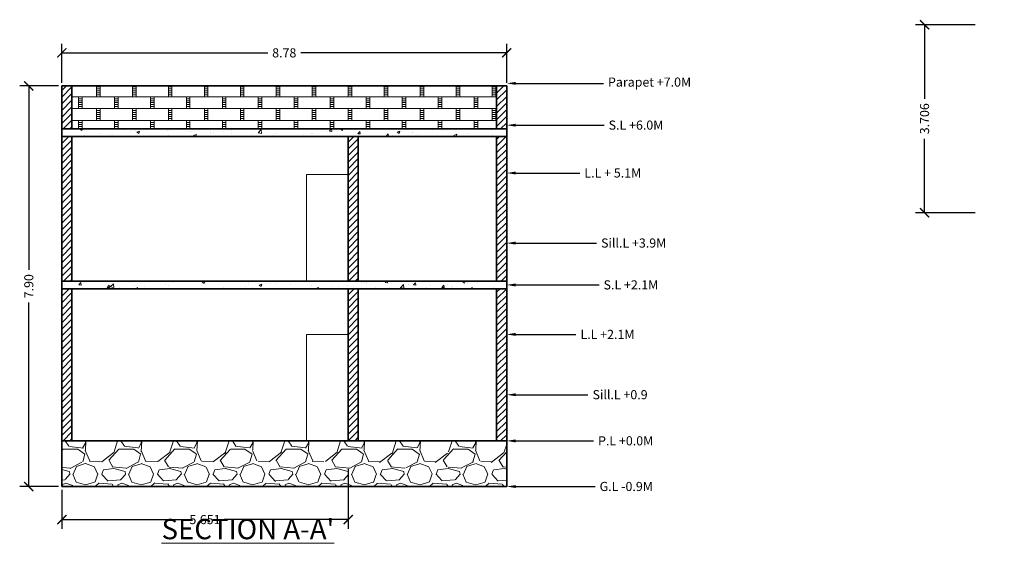
# Model space of a CAD drawing. Units: metres. Extents: x 6.8 to 74, y 0.6 to 37.
# Tile 4 of 5: x 20.7 to 40.1, y 19.5 to 29.9. Entities that reach past the tile are written whole.
import ezdxf
from ezdxf import colors
from ezdxf.entities.mleader import LeaderData, LeaderLine
from ezdxf.math import Vec2, Vec3

# ---------------------------------------------------------------- set-up
doc = ezdxf.new("R2010")
doc.units = ezdxf.units.M
doc.header["$LTSCALE"] = 0.2
doc.header["$MEASUREMENT"] = 0
for name, color, linetype, lineweight in [('A-ANNO-DIMS', 2, 'Continuous', 18), ('A-ANNO-SYMB', 3, 'Continuous', 18), ('A-ANNO-TEXT', 7, 'Continuous', 18), ('A-DOOR', 4, 'Continuous', 20), ('A-SECT', 7, 'Continuous', 35), ('A-SECT-PATT', 252, 'Continuous', 13)]:
    doc.layers.add(name, color=color, linetype=linetype, lineweight=lineweight)
doc.styles.get("Standard").update_dxf_attribs({"font": 'arial.ttf'})
doc.dimstyles.get("Standard").update_dxf_attribs({"dimtxt": 0.18, "dimasz": 0.18, "dimexe": 0.18, "dimexo": 0.0625, "dimgap": 0.09, "dimtad": 0, "dimzin": 0, "dimdsep": 46, "dimtxsty": 'Standard', "dimblk": 'ARCHTICK', "dimcen": 0.09, "dimadec": 0, "dimazin": 0, "dimtfac": 1, "dimtofl": 0, "dimtmove": 0, "dimatfit": 3, "dimfxl": 1, "dimfxlon": 1, "dimtolj": 1, "dimtzin": 0, "dimarcsym": 0})
pattern_1 = [(45, (0, 0), (-0.0654073772597557, 0.0654073772597557), [])]

# ---------------------------------------------------------------- blocks, each defined once
blk = doc.blocks.new('_ArchTick')
at = {"color": 0, "linetype": 'ByBlock', "const_width": 0.15}
blk.add_lwpolyline([(-0.5, -0.5), (0.5, 0.5)], dxfattribs=at)
blk = doc.blocks.new('*D56')
at = {"layer": 'A-ANNO-DIMS', "color": 0, "lineweight": -2, "ltscale": 0.9, "transparency": 16777216}
for p, q in [((21.540083, 28.626551), (21.540083, 29.395551)), ((30.320083, 28.626551), (30.320083, 29.395551)), ((21.540083, 29.215551), (25.60599705184175, 29.215551)), ((30.320083, 29.215551), (26.25416894815825, 29.215551))]:
    blk.add_line(p, q, dxfattribs=at)
at = {"layer": 'Defpoints', "color": 0, "ltscale": 0.9, "transparency": 16777216}
for p in [(30.320083, 29.215551), (21.540083, 28.564051), (30.320083, 28.564051)]:
    blk.add_point(p, dxfattribs=at)
at = {"layer": 'A-ANNO-DIMS', "color": 0, "lineweight": -2, "ltscale": 0.9, "transparency": 16777216, "xscale": 0.18, "yscale": 0.18, "zscale": 0.18, "rotation": 180}
blk.add_blockref('_ArchTick', (21.540083, 29.215551), dxfattribs=at)
at = {"layer": 'A-ANNO-DIMS', "color": 0, "lineweight": -2, "ltscale": 0.9, "transparency": 16777216, "xscale": 0.18, "yscale": 0.18, "zscale": 0.18}
blk.add_blockref('_ArchTick', (30.320083, 29.215551), dxfattribs=at)
at = {"layer": 'A-ANNO-DIMS', "color": 0, "ltscale": 0.9, "transparency": 16777216, "insert": (25.930083, 29.215551), "char_height": 0.18, "attachment_point": 5}
blk.add_mtext('\\A1;8.78', dxfattribs=at)
blk = doc.blocks.new('*D57')
at = {"layer": 'A-ANNO-DIMS', "color": 0, "lineweight": -2, "ltscale": 0.9, "transparency": 16777216}
for p, q in [((21.47758300000001, 28.56405100000002), (20.70858300000002, 28.56405100000002)), ((20.88858300000001, 28.56405100000002), (20.88858300000001, 24.93678633424285)), ((20.88858300000002, 20.66405100000001), (20.88858300000001, 24.29131566575718)), ((21.47758300000001, 20.66405100000001), (20.70858300000002, 20.66405100000001))]:
    blk.add_line(p, q, dxfattribs=at)
at = {"layer": 'Defpoints', "color": 0, "ltscale": 0.9, "transparency": 16777216}
for p in [(20.88858300000001, 28.56405100000002), (21.540083, 28.56405100000002), (21.540083, 20.66405100000001)]:
    blk.add_point(p, dxfattribs=at)
at = {"layer": 'A-ANNO-DIMS', "color": 0, "lineweight": -2, "ltscale": 0.9, "transparency": 16777216, "xscale": 0.18, "yscale": 0.18, "zscale": 0.18}
for p, rotation in [((20.88858300000001, 28.56405100000002), 90), ((20.88858300000002, 20.66405100000001), 270)]:
    blk.add_blockref('_ArchTick', p, dxfattribs=dict(at, rotation=rotation))
at = {"layer": 'A-ANNO-DIMS', "color": 0, "ltscale": 0.9, "transparency": 16777216, "insert": (20.88858300000002, 24.614051), "char_height": 0.18, "attachment_point": 5, "rotation": 90}
blk.add_mtext('\\A1;7.90', dxfattribs=at)
blk = doc.blocks.new('*D58')
at = {"layer": 'A-ANNO-DIMS', "color": 0, "lineweight": -2, "ltscale": 0.9, "transparency": 16777216}
for p, q in [((27.190671, 21.012551), (27.190671, 19.832551)), ((21.540083, 20.601551), (21.540083, 19.832551)), ((21.540083, 20.012551), (23.98904684993178, 20.012551)), ((27.190671, 20.012551), (24.74170715006821, 20.012551))]:
    blk.add_line(p, q, dxfattribs=at)
at = {"layer": 'Defpoints', "color": 0, "ltscale": 0.9, "transparency": 16777216}
for p in [(27.190671, 21.564051), (21.540083, 20.664051), (27.190671, 20.012551)]:
    blk.add_point(p, dxfattribs=at)
at = {"layer": 'A-ANNO-DIMS', "color": 0, "lineweight": -2, "ltscale": 0.9, "transparency": 16777216, "xscale": 0.18, "yscale": 0.18, "zscale": 0.18, "rotation": 180}
blk.add_blockref('_ArchTick', (21.540083, 20.012551), dxfattribs=at)
at = {"layer": 'A-ANNO-DIMS', "color": 0, "lineweight": -2, "ltscale": 0.9, "transparency": 16777216, "xscale": 0.18, "yscale": 0.18, "zscale": 0.18}
blk.add_blockref('_ArchTick', (27.190671, 20.012551), dxfattribs=at)
at = {"layer": 'A-ANNO-DIMS', "color": 0, "ltscale": 0.9, "transparency": 16777216, "insert": (24.365377, 20.012551), "char_height": 0.18, "attachment_point": 5}
blk.add_mtext('\\A1;5.651', dxfattribs=at)
blk = doc.blocks.new('*D61')
at = {"layer": 'A-ANNO-DIMS', "color": 0, "lineweight": -2, "ltscale": 0.9, "transparency": 16777216}
for p, q in [((39.56668000000003, 29.76942700000001), (38.38668000000003, 29.76942700000001)), ((38.56668000000003, 29.76942700000001), (38.56668000000003, 28.30996317326059)), ((38.56668000000003, 26.06333700000001), (38.56668000000003, 27.52280082673944)), ((39.56668000000003, 26.06333700000001), (38.38668000000003, 26.06333700000001))]:
    blk.add_line(p, q, dxfattribs=at)
at = {"layer": 'Defpoints', "color": 0, "ltscale": 0.9, "transparency": 16777216}
for p in [(38.56668000000003, 29.76942700000001), (52.66698100000002, 29.76942700000002), (52.66698100000002, 26.06333700000002)]:
    blk.add_point(p, dxfattribs=at)
at = {"layer": 'A-ANNO-DIMS', "color": 0, "lineweight": -2, "ltscale": 0.9, "transparency": 16777216, "xscale": 0.18, "yscale": 0.18, "zscale": 0.18}
for p, rotation in [((38.56668000000003, 29.76942700000001), 90), ((38.56668000000003, 26.06333700000001), 270)]:
    blk.add_blockref('_ArchTick', p, dxfattribs=dict(at, rotation=rotation))
at = {"layer": 'A-ANNO-DIMS', "color": 0, "ltscale": 0.9, "transparency": 16777216, "insert": (38.56668000000003, 27.91638199999999), "char_height": 0.18, "attachment_point": 5, "rotation": 90}
blk.add_mtext('\\A1;3.706', dxfattribs=at)

msp = doc.modelspace()

# ---------------------------------------------------------------- hatches: boundary and pattern name
at = {"layer": 'A-SECT-PATT'}
h = msp.add_hatch(dxfattribs=at)
h.set_pattern_fill('ANSI31', color=256, scale=0.7400000000000001)
h.set_pattern_definition(pattern_1)
h.paths.add_polyline_path([(21.7400830914722, 27.56405142054635), (21.5400830914722, 27.56405142054635), (21.5400830914722, 24.71405142054635), (21.7400830914722, 24.71405142054635)])
h.paths.add_polyline_path([(21.7400830914722, 28.56405142054635), (21.5400830914722, 28.56405142054635), (21.5400830914722, 27.71405142054635), (21.7400830914722, 27.71405142054635)])
h.paths.add_polyline_path([(30.32008309147219, 28.56405142054635), (30.1200830914722, 28.56405142054635), (30.1200830914722, 27.71405142054635), (30.3200830914722, 27.71405142054635)])
h.paths.add_polyline_path([(30.3200830914722, 27.56405142054635), (30.1200830914722, 27.56405142054635), (30.1200830914722, 24.71405142054635), (30.3200830914722, 24.71405142054635)])
h.paths.add_polyline_path([(21.7400830914722, 24.56405142054635), (21.5400830914722, 24.56405142054635), (21.5400830914722, 21.56405142054635), (21.7400830914722, 21.56405142054635)])
h.paths.add_polyline_path([(30.3200830914722, 24.56405142054635), (30.1200830914722, 24.56405142054635), (30.1200830914722, 21.56405142054635), (30.3200830914722, 21.56405142054635)])
h = msp.add_hatch(dxfattribs=at)
h.set_pattern_fill('BRSTONE', color=256, scale=0.71)
h.set_pattern_definition([(0, (0, 0), (0, 0.2343), []), (90, (0.6390000000000001, 0), (-0.355, 0.2343), [0.2343, -0.2343]), (90, (0.568, 0), (-0.355, 0.2343), [0.2343, -0.2343]), (0, (0.6390000000000001, 0.03905), (0.355, 0.2343), [-0.6390000000000001, 0.071]), (0, (0.6390000000000001, 0.0781), (0.355, 0.2343), [-0.6390000000000001, 0.071]), (0, (0.6390000000000001, 0.11715), (0.355, 0.2343), [-0.6390000000000001, 0.071]), (0, (0.6390000000000001, 0.1562), (0.355, 0.2343), [-0.6390000000000001, 0.071]), (0, (0.6390000000000001, 0.19525), (0.355, 0.2343), [-0.6390000000000001, 0.071])])
h.paths.add_polyline_path([(30.1200830914722, 28.56405142054635), (21.7400830914722, 28.56405142054635), (21.7400830914722, 27.71405142054635), (30.1200830914722, 27.71405142054635)])
h = msp.add_hatch(dxfattribs=at)
h.set_pattern_fill('AR-CONC', color=256, scale=0.078)
h.set_pattern_definition([(50, (0, 0), (0.5594629424285877, -0.0489466652864242), [0.0585, -0.6435]), (355, (0, 0), (-0.10822604021814, 0.5867098642860094), [0.0468, -0.5148]), (100.45144446, (0.04662191118, -0.00407888832), (0.4512369004471474, 0.537763192955531), [0.04971734976, -0.5468908473599999]), (46.1842, (0, 0.156), (0.8324482379238265, -0.1291050390185997), [0.08775, -0.9652499999999999]), (96.63563549000003, (0.0693706611, 0.14524122054), (0.7290363176258982, 0.7598125086041494), [0.07457606676, -0.8203367327999997]), (351.18416399, (0, 0.156), (0.729036317142723, 0.7598125082105924), [0.0702, -0.77220000078]), (21, (0.078, 0.117), (0.4655875006524001, -0.3140427347189643), [0.0585, -0.6435]), (326, (0.078, 0.117), (0.1897859588988337, 0.5656170351365454), [0.0468, -0.5148]), (71.45144474, (0.11679895812, 0.09082977228), (0.6553734538493776, 0.251574299188956), [0.0497173482, -0.5468908473599999]), (37.5, (0, 0), (0.0094846871474867, 0.259657205988423), [0, -0.5085600000000001, 0, -0.5226000000000001, 0, -0.5167500000000002]), (7.499999999999999, (0, 0), (0.2051942392048759, 0.307641135268241), [0, -0.29796, 0, -0.4968600000000001, 0, -0.19695]), (327.5, (-0.17394, 0), (0.416381500214479, -0.0175927999528162), [0, -0.195, 0, -0.6084, 0, -0.8073]), (317.5, (-0.25194, 0), (0.4548852120870614, 0.0780818862192078), [0, -0.2535, 0, -0.40404, 0, -0.5732999999999999])])
h.paths.add_polyline_path([(30.3200830914722, 27.71405142054635), (21.5400830914722, 27.71405142054635), (21.5400830914722, 27.56405142054635), (30.3200830914722, 27.56405142054635)])
h.paths.add_polyline_path([(30.3200830914722, 24.71405142054635), (21.5400830914722, 24.71405142054635), (21.5400830914722, 24.56405142054635), (30.3200830914722, 24.56405142054635)])
h = msp.add_hatch(dxfattribs=at)
h.set_pattern_fill('ANSI31', color=256, scale=0.7400000000000001)
h.set_pattern_definition(pattern_1)
h.paths.add_polyline_path([(27.39067071819349, 27.56405142054635), (27.19067071819349, 27.56405142054635), (27.19067071819349, 24.71405142054635), (27.39067071819349, 24.71405142054635)])
h.paths.add_polyline_path([(27.39067071819349, 24.56405142054635), (27.19067071819349, 24.56405142054635), (27.19067071819349, 21.56405142054635), (27.39067071819349, 21.56405142054635)])
h = msp.add_hatch(dxfattribs=at)
h.set_pattern_fill('GRAVEL', color=256, scale=1.099999999999999)
h.set_pattern_definition([(228.012787504, (0.7919999999999999, 1.099999999999999), (-8.800000000000066, -9.900000000000002), [0.1479896, -14.65099685178106]), (184.969740728, (0.693, 0.9899999999999998), (13.19999999999997, 1.100000000000038), [0.2539548, -25.14151723735299]), (132.510447078, (0.44, 0.9679999999999997), (11.00000000000012, -12.09999999999985), [0.1790668, -17.72763585570967]), (267.273689006, (0.011, 0.693), (1.100000000000026, 22.00000000000002), [0.2312618, -22.89491384579189]), (292.833654178, (0, 0.462), (-5.499999999999986, 13.20000000000003), [0.2267704999999999, -22.45031044089713]), (357.273689006, (0.088, 0.253), (-22.00000000000002, 1.100000000000027), [0.2312618, -22.89491384579189]), (37.6942404667, (0.3189999999999999, 0.2419999999999999), (-14.29999999999999, -10.99999999999997), [0.3058318999999999, -30.2773334038076]), (72.2553283749, (0.561, 0.429), (7.700000000000029, 24.2), [0.2887367999999999, -28.58495364649473]), (121.429565615, (0.649, 0.704), (-8.80000000000002, 14.29999999999998), [0.232045, -22.9724804207019]), (175.236358309, (0.528, 0.9019999999999997), (12.09999999999998, -1.100000000000041), [0.2649151999999999, -12.98083883667153]), (222.397437798, (0.264, 0.9239999999999998), (-13.19999999999996, -12.09999999999997), [0.3425928, -33.91671250527438]), (138.814074834, (1.099999999999999, 0.682), (-7.700000000000034, 6.599999999999999), [0.1169311, -11.57622929400816]), (171.46923439, (1.012, 0.7589999999999999), (14.29999999999999, -2.199999999999994), [0.2224607, -22.0236625577727]), (225, (0.7919999999999999, 0.7919999999999999), (-1e-16, -1.099999999999926), [0.1555631, -1.400071818610409]), (203.198590514, (0.715, 0.9239999999999998), (5.499999999999987, 2.199999999999972), [0.0837738, -8.29357661645029]), (291.801409486, (0.6379999999999999, 0.8909999999999998), (-1.099999999999652, 3.300000000000112), [0.1184733, -5.805207987847949]), (30.96375653209999, (0.682, 0.7809999999999999), (3.300000000000057, 2.199999999999977), [0.1924219, -6.221625184329828]), (161.565051177, (0.8469999999999998, 0.8799999999999998), (2.200000000000012, -1.099999999999974), [0.1391401, -3.339365326185238]), (16.389540334, (0, 0.8909999999999998), (10.99999999999996, 3.300000000000047), [0.19492, -19.29712966133634]), (70.3461759419, (0.187, 0.946), (-4.400000000001341, -12.10000000000373), [0.1635270999999999, -16.18914852205089]), (293.198590514, (0.8469999999999998, 1.099999999999999), (-2.199999999999967, 5.499999999999989), [0.1675465, -8.209803916450287]), (343.610459666, (0.9129999999999999, 0.946), (-10.99999999999996, 3.300000000000047), [0.19492, -19.29712966133589]), (339.44395478, (0, 0.209), (-5.500000000000039, 2.200000000000026), [0.1879679999999999, -9.210436119849247]), (294.775140569, (0.176, 0.143), (-5.500000000000005, 12.1), [0.1574958, -15.5921073696036]), (66.8014094864, (0.8579999999999998, 0), (2.199999999999978, 5.499999999999966), [0.1675465, -8.209803916450287]), (17.3540246363, (0.9239999999999998, 0.154), (-14.29999999999997, -4.399999999999958), [0.1843941, -18.254965975664]), (69.4439547804, (0.3189999999999999, 0), (-2.200000000000007, -5.499999999999949), [0.093984, -9.304420119849247]), (101.309932474, (0.7919999999999999, 0), (-1.09999999999996, 4.400000000000012), [0.056089, -5.552832464952079]), (165.963756532, (0.7809999999999999, 0.055), (3.299999999999954, -1.100000000000001), [0.2267705, -4.30864568817947]), (186.009005957, (0.561, 0.11), (11.00000000000005, 1.099999999999981), [0.210155, -20.80531549199708]), (303.690067526, (0.682, 0.682), (-1.099999999999985, 2.199999999999984), [0.1586441999999999, -3.807462203010399]), (353.157226587, (0.77, 0.55), (18.70000000000001, -2.200000000000057), [0.2769734, -27.42031888643113]), (60.9453959009, (1.044999999999999, 0.5169999999999999), (-4.399999999999972, -7.699999999999973), [0.1132516, -11.2119415550857]), (90, (1.099999999999999, 0.6160000000000001), (-1.099999999999999, 1.099999999999999), [0.066, -1.033999999999999]), (120.256437164, (0.5389999999999999, 0.143), (4.400000000000009, -7.700000000000008), [0.1528164, -15.12887198839478]), (48.01278750419999, (0.462, 0.275), (8.799999999999997, 9.89999999999997), [0.2959791999999999, -14.50300725178106]), (0, (0.66, 0.495), (1.099999999999999, 1.099999999999999), [0.286, -0.8139999999999998]), (325.304846469, (0.946, 0.495), (11.00000000000015, -7.699999999999806), [0.1739253999999999, -17.21860173092619]), (254.0546040990001, (1.088999999999999, 0.3959999999999999), (-1.100000000000041, -4.400000000000003), [0.1601622, -7.847958678208549]), (207.645975364, (1.044999999999999, 0.2419999999999999), (-20.89999999999994, -11.00000000000005), [0.2607715, -25.81642160048533]), (175.42607874, (0.8139999999999998, 0.121), (-14.29999999999995, 1.100000000000001), [0.2758789, -27.31198074876579])])
h.paths.add_polyline_path([(30.3200830914722, 21.56405142054635), (21.5400830914722, 21.56405142054635), (21.5400830914722, 20.66405142054635), (30.3200830914722, 20.66405142054635)])

# ---------------------------------------------------------------- linework, layer by layer
at = {"layer": 'A-DOOR'}
for points in [[(27.19067071819349, 26.81405142054635), (26.36950474556888, 26.81405142054635), (26.36950474556888, 24.71405142054635), (27.19067071819349, 24.71405142054635)], [(27.19067071819349, 23.66405142054635), (26.36950474556888, 23.66405142054635), (26.36950474556888, 21.56405142054635), (27.19067071819349, 21.56405142054635)]]:
    msp.add_lwpolyline(points, close=True, dxfattribs=at)
at = {"layer": 'A-SECT'}
for p, q in [((21.5400830914722, 28.56405142054635), (30.3200830914722, 28.56405142054635)), ((21.5400830914722, 27.56405142054635), (21.5400830914722, 28.56405142054635)), ((21.7400830914722, 27.71405142054635), (21.7400830914722, 28.56405142054635)), ((30.1200830914722, 28.56405142054635), (30.1200830914722, 27.71405142054635)), ((30.3200830914722, 28.56405142054635), (30.3200830914722, 27.56405142054636)), ((21.5400830914722, 27.71405142054635), (30.3200830914722, 27.71405142054635)), ((21.5400830914722, 27.56405142054635), (30.3200830914722, 27.56405142054635)), ((21.5400830914722, 24.71405142054635), (21.5400830914722, 27.56405142054635)), ((21.7400830914722, 24.71405142054635), (21.7400830914722, 27.56405142054635)), ((27.19067071819349, 24.71405142054635), (27.19067071819349, 27.56405142054636)), ((27.39067071819349, 24.71405142054635), (27.39067071819349, 27.56405142054636)), ((30.1200830914722, 27.56405142054636), (30.1200830914722, 24.71405142054635)), ((30.3200830914722, 27.56405142054636), (30.3200830914722, 24.71405142054635)), ((21.5400830914722, 24.71405142054635), (30.3200830914722, 24.71405142054635)), ((21.5400830914722, 24.56405142054635), (21.5400830914722, 24.71405142054635)), ((30.3200830914722, 24.71405142054635), (30.3200830914722, 24.56405142054635)), ((21.5400830914722, 24.56405142054635), (30.3200830914722, 24.56405142054635)), ((21.5400830914722, 21.56405142054635), (21.5400830914722, 24.56405142054635)), ((21.7400830914722, 21.56405142054635), (21.7400830914722, 24.56405142054635)), ((27.19067071819349, 21.56405142054635), (27.19067071819349, 24.56405142054635)), ((27.39067071819349, 21.56405142054635), (27.39067071819349, 24.56405142054635)), ((30.1200830914722, 24.56405142054635), (30.1200830914722, 21.56405142054635)), ((30.3200830914722, 24.56405142054635), (30.3200830914722, 21.56405142054635)), ((21.5400830914722, 21.56405142054635), (30.3200830914722, 21.56405142054635)), ((21.5400830914722, 20.66405142054635), (21.5400830914722, 21.56405142054635)), ((30.3200830914722, 21.56405142054635), (30.3200830914722, 20.66405142054635)), ((21.5400830914722, 20.66405142054635), (30.3200830914722, 20.66405142054635))]:
    msp.add_line(p, q, dxfattribs=at)

# ---------------------------------------------------------------- texts
at = {"layer": 'A-ANNO-TEXT', "insert": (23.50848088502431, 20.02505097242608), "char_height": 0.4, "attachment_point": 1}
msp.add_mtext_dynamic_manual_height_columns("{\\LSECTION A-A'}", width=7.004507583875465, gutter_width=1, heights=[0], dxfattribs=at)

# ---------------------------------------------------------------- dimensions: what is measured, and where the dimension line sits
at = {"layer": 'A-ANNO-DIMS', "ltscale": 0.9}
for base, p1, p2, override, picture, middle in [((38.56668000000003, 29.76942700000001), (52.666981, 26.063337), (52.666981, 29.769427), {"dimdec": 3, "dimlfac": 1, "dimrnd": 0, "dimzin": 0, "dimdsep": 46, "dimlunit": 2}, '*D61', (38.56668000000003, 27.91638199999999)), ((20.88858300000001, 28.56405100000002), (21.540083, 20.664051), (21.540083, 28.564051), {"dimdec": 2, "dimlfac": 1, "dimrnd": 0, "dimzin": 0, "dimdsep": 46, "dimlunit": 2}, '*D57', (20.88858300000002, 24.614051))]:
    dim = msp.add_linear_dim(base=base, p1=p1, p2=p2, angle=90, dimstyle='Standard', override=override, dxfattribs=at)
    dim.commit()
    dim.dimension.update_dxf_attribs({"geometry": picture, "text_midpoint": middle})
for base, p1, p2, override, picture, middle in [((30.320083, 29.215551), (21.540083, 28.564051), (30.320083, 28.564051), {"dimdec": 2, "dimlfac": 1, "dimrnd": 0, "dimzin": 0, "dimdsep": 46, "dimlunit": 2}, '*D56', (25.930083, 29.215551)), ((27.190671, 20.012551), (21.540083, 20.664051), (27.190671, 21.564051), {"dimdec": 3, "dimlfac": 1, "dimrnd": 0, "dimzin": 0, "dimdsep": 46, "dimlunit": 2}, '*D58', (24.365377, 20.012551))]:
    dim = msp.add_linear_dim(base=base, p1=p1, p2=p2, dimstyle='Standard', override=override, dxfattribs=at)
    dim.commit()
    dim.dimension.update_dxf_attribs({"geometry": picture, "text_midpoint": middle})

# ---------------------------------------------------------------- leaders
at = {"layer": 'A-ANNO-SYMB'}
ml = msp.add_multileader_mtext('Standard', dxfattribs=at)
ml.set_content('Parapet +7.0M', color=256)
ml.set_leader_properties()
ml.build(insert=Vec2(0, 0))
ml.multileader.update_dxf_attribs({"dogleg_length": 0.36, "arrow_head_size": 0.18})
ctx = ml.context
ctx.base_point, ctx.char_height, ctx.arrow_head_size, ctx.landing_gap_size, ctx.plane_origin = Vec3(32.22950831367833, 28.61405142054635), 0.18, 0.18, 0.09, Vec3(30.3200830914722, 28.61405142054635)
notes = []
notes.append((ctx, [(0, (1, 1, 0), (31.86950831367833, 28.61405142054635), (1, 0), 0.36, [(0, [(30.3200830914722, 28.61405142054635)], 0, [])])]))
ctx.mtext.insert, ctx.mtext.flow_direction = Vec3(32.31950831367833, 28.72903777798154), 5
ml = msp.add_multileader_mtext('Standard', dxfattribs=at)
ml.set_content('S.L +6.0M', color=256)
ml.set_leader_properties()
ml.build(insert=Vec2(0, 0))
ml.multileader.update_dxf_attribs({"dogleg_length": 0.36, "arrow_head_size": 0.18})
ctx = ml.context
ctx.base_point, ctx.char_height, ctx.arrow_head_size, ctx.landing_gap_size, ctx.plane_origin = Vec3(32.24191849951711, 27.78905142054635), 0.18, 0.18, 0.09, Vec3(30.3200830914722, 27.78905142054635)
notes.append((ctx, [(0, (1, 1, 0), (31.88191849951711, 27.78905142054635), (1, 0), 0.36, [(0, [(30.3200830914722, 27.78905142054635)], 0, [])])]))
ctx.mtext.insert, ctx.mtext.flow_direction = Vec3(32.3319184995171, 27.88058620908659), 5
ml = msp.add_multileader_mtext('Standard', dxfattribs=at)
ml.set_content('L.L + 5.1M', color=256)
ml.set_leader_properties()
ml.build(insert=Vec2(0, 0))
ml.multileader.update_dxf_attribs({"dogleg_length": 0.36, "arrow_head_size": 0.18})
ctx = ml.context
ctx.base_point, ctx.char_height, ctx.arrow_head_size, ctx.landing_gap_size, ctx.plane_origin = Vec3(31.763273493009, 26.845742130509), 0.18, 0.18, 0.09, Vec3(30.3200830914722, 26.845742130509)
notes.append((ctx, [(0, (1, 1, 0), (31.403273493009, 26.845742130509), (1, 0), 0.36, [(0, [(30.3200830914722, 26.845742130509)], 0, [])])]))
ctx.mtext.insert, ctx.mtext.flow_direction = Vec3(31.853273493009, 26.93727691904925), 5
ml = msp.add_multileader_mtext('Standard', dxfattribs=at)
ml.set_content('Sill.L +3.9M', color=256)
ml.set_leader_properties()
ml.build(insert=Vec2(0, 0))
ml.multileader.update_dxf_attribs({"dogleg_length": 0.36, "arrow_head_size": 0.18})
ctx = ml.context
ctx.base_point, ctx.char_height, ctx.arrow_head_size, ctx.landing_gap_size, ctx.plane_origin = Vec3(32.09262612318314, 25.46405142054635), 0.18, 0.18, 0.09, Vec3(30.3200830914722, 25.46405142054635)
notes.append((ctx, [(0, (1, 1, 0), (31.73262612318314, 25.46405142054635), (1, 0), 0.36, [(0, [(30.3200830914722, 25.46405142054635)], 0, [])])]))
ctx.mtext.insert, ctx.mtext.flow_direction = Vec3(32.18262612318314, 25.5556476006282), 5
ml = msp.add_multileader_mtext('Standard', dxfattribs=at)
ml.set_content('S.L +2.1M', color=256)
ml.set_leader_properties()
ml.build(insert=Vec2(0, 0))
ml.multileader.update_dxf_attribs({"dogleg_length": 0.36, "arrow_head_size": 0.18})
ctx = ml.context
ctx.base_point, ctx.char_height, ctx.arrow_head_size, ctx.landing_gap_size, ctx.plane_origin = Vec3(32.14226183151319, 24.63905142054635), 0.18, 0.18, 0.09, Vec3(30.3200830914722, 24.63905142054635)
notes.append((ctx, [(0, (1, 1, 0), (31.78226183151318, 24.63905142054635), (1, 0), 0.36, [(0, [(30.3200830914722, 24.63905142054635)], 0, [])])]))
ctx.mtext.insert, ctx.mtext.flow_direction = Vec3(32.23226183151318, 24.7305862090866), 5
ml = msp.add_multileader_mtext('Standard', dxfattribs=at)
ml.set_content('L.L +2.1M', color=256)
ml.set_leader_properties()
ml.build(insert=Vec2(0, 0))
ml.multileader.update_dxf_attribs({"dogleg_length": 0.36, "arrow_head_size": 0.18})
ctx = ml.context
ctx.base_point, ctx.char_height, ctx.arrow_head_size, ctx.landing_gap_size, ctx.plane_origin = Vec3(31.68594931888583, 23.66405142054635), 0.18, 0.18, 0.09, Vec3(30.3200830914722, 23.66405142054635)
notes.append((ctx, [(0, (1, 1, 0), (31.32594931888583, 23.66405142054635), (1, 0), 0.36, [(0, [(30.3200830914722, 23.66405142054635)], 0, [])])]))
ctx.mtext.insert, ctx.mtext.flow_direction = Vec3(31.77594931888583, 23.75411281208796), 5
ml = msp.add_multileader_mtext('Standard', dxfattribs=at)
ml.set_content('Sill.L +0.9', color=256)
ml.set_leader_properties()
ml.build(insert=Vec2(0, 0))
ml.multileader.update_dxf_attribs({"dogleg_length": 0.36, "arrow_head_size": 0.18})
ctx = ml.context
ctx.base_point, ctx.char_height, ctx.arrow_head_size, ctx.landing_gap_size, ctx.plane_origin = Vec3(31.92416742056584, 22.47386303570537), 0.18, 0.18, 0.09, Vec3(30.3200830914722, 22.47386303570537)
notes.append((ctx, [(0, (1, 1, 0), (31.56416742056584, 22.47386303570537), (1, 0), 0.36, [(0, [(30.3200830914722, 22.47386303570537)], 0, [])])]))
ctx.mtext.insert, ctx.mtext.flow_direction = Vec3(32.01416742056584, 22.56539782424562), 5
ml = msp.add_multileader_mtext('Standard', dxfattribs=at)
ml.set_content('P.L +0.0M', color=256)
ml.set_leader_properties()
ml.build(insert=Vec2(0, 0))
ml.multileader.update_dxf_attribs({"dogleg_length": 0.36, "arrow_head_size": 0.18})
ctx = ml.context
ctx.base_point, ctx.char_height, ctx.arrow_head_size, ctx.landing_gap_size, ctx.plane_origin = Vec3(32.03342818302977, 21.56405142054635), 0.18, 0.18, 0.09, Vec3(30.3200830914722, 21.56405142054635)
notes.append((ctx, [(0, (1, 1, 0), (31.67342818302976, 21.56405142054635), (1, 0), 0.36, [(0, [(30.3200830914722, 21.56405142054635)], 0, [])])]))
ctx.mtext.insert, ctx.mtext.flow_direction = Vec3(32.12342818302976, 21.65558620908659), 5
ml = msp.add_multileader_mtext('Standard', dxfattribs=at)
ml.set_content('G.L -0.9M', color=256)
ml.set_leader_properties()
ml.build(insert=Vec2(0, 0))
ml.multileader.update_dxf_attribs({"dogleg_length": 0.36, "arrow_head_size": 0.18})
ctx = ml.context
ctx.base_point, ctx.char_height, ctx.arrow_head_size, ctx.landing_gap_size, ctx.plane_origin = Vec3(32.06328732004271, 20.66405142054635), 0.18, 0.18, 0.09, Vec3(30.3200830914722, 20.66405142054635)
notes.append((ctx, [(0, (1, 1, 0), (31.70328732004271, 20.66405142054635), (1, 0), 0.36, [(0, [(30.3200830914722, 20.66405142054635)], 0, [])])]))
ctx.mtext.insert, ctx.mtext.flow_direction = Vec3(32.15328732004271, 20.7555862090866), 5
for ctx, leaders in notes:
    for number, flags, end, landing, length, lines in leaders:
        leader = LeaderData()
        leader.index, (leader.has_last_leader_line, leader.has_dogleg_vector, leader.attachment_direction) = number, flags
        leader.last_leader_point, leader.dogleg_vector, leader.dogleg_length = Vec3(end), Vec3(landing), length
        for number, points, colour, breaks in lines:
            line = LeaderLine()
            line.index, line.vertices, line.color, line.breaks = number, Vec3.list(points), colors.encode_raw_color(colour), breaks
            leader.lines.append(line)
        ctx.leaders.append(leader)

doc.saveas('drawing.dxf')
